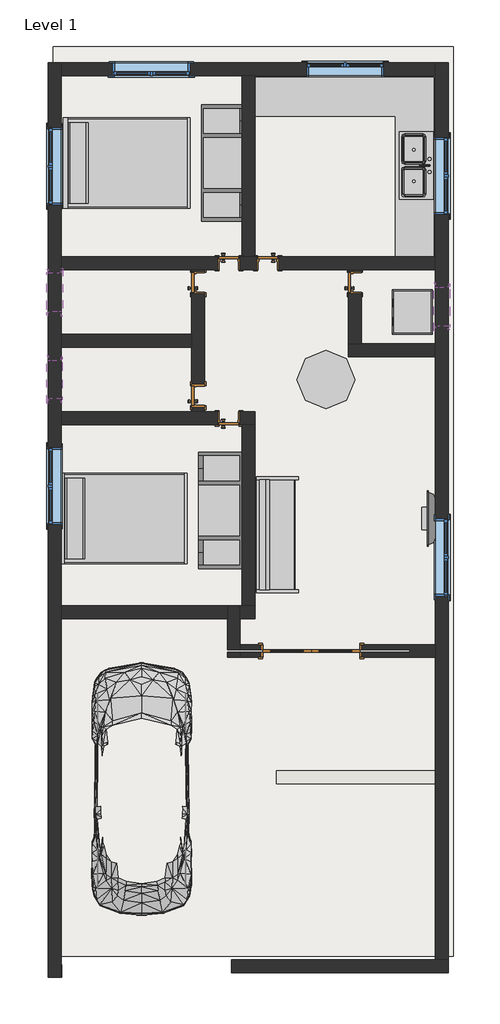
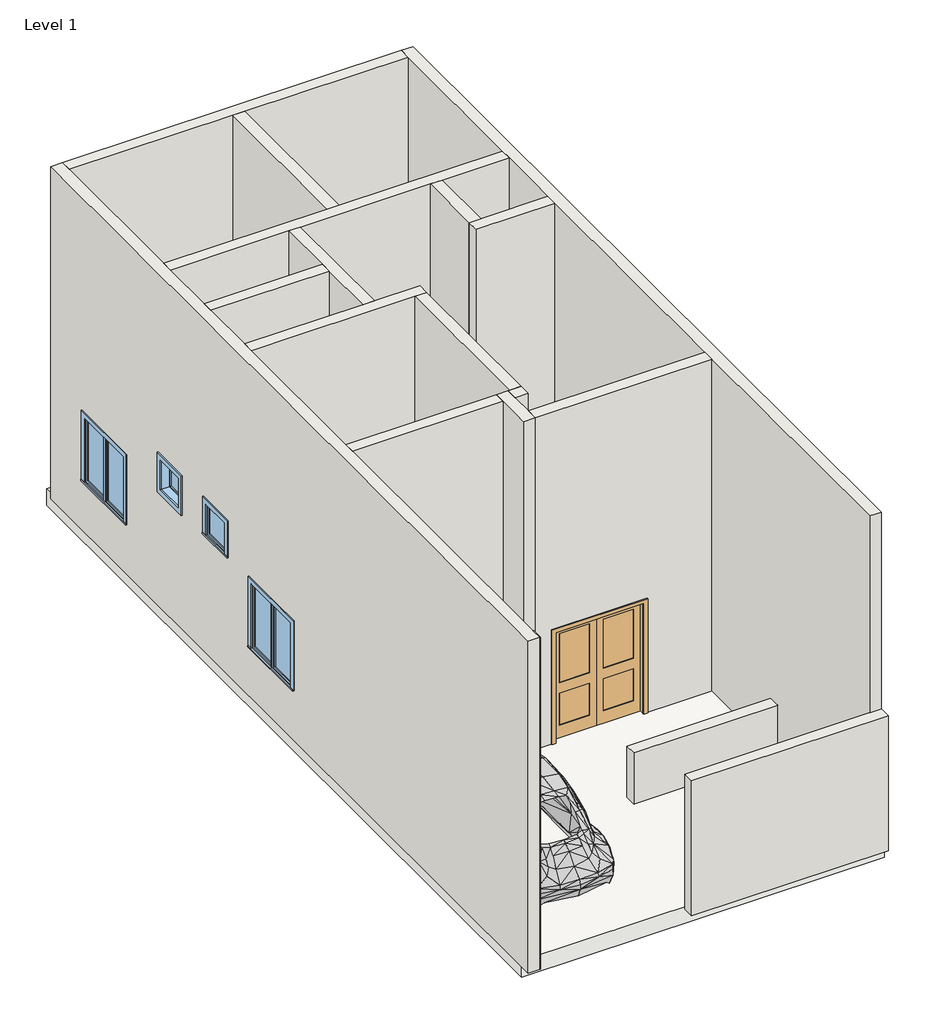
# One storey, incomplete: 17 walls, 9 windows, 8 furniture elements, 7 doors, 2 proxies, 1 flow terminal, 1 slab.
"""IFC4 building model written with IfcOpenShell, lengths in millimetres."""

from ifc_helpers import new_model, si_unit, frame, origin, origin_with_axes, place, context, project, spatial, polyline, outline, extrude, faceted_brep, transform, mapped, element, save
from components import rpc_beetle_rpc_beetle_3ce7ba48, recycle_bin_square_recycle_bin_square_c944da42, door_4110a08e, door_6ef897ee, door_5a382651, door_b2d2822a, flow_terminal_a53be723, furniture_096e7f55, furniture_8bbd1b1f, furniture_cf0b6580, furniture_a4ffab56, furniture_56245f3a, furniture_905aceb5, window_0862ab64, window_e41d21a6

model = new_model("IFC4")

# Units and contexts
model_context = context("Model", 3, world=origin())
ifc_project = project(units=[si_unit("LENGTHUNIT", "METRE", prefix="MILLI")], contexts=[model_context])

# Site, building, storey
site = spatial("IfcSite", under=ifc_project)
building = spatial("IfcBuilding", under=site)
storey = spatial("IfcBuildingStorey", under=building, Name="Level 1", Elevation=0.0)

# Proxies
placement = place(None, origin())
rpc_beetle_rpc_beetle_shape = rpc_beetle_rpc_beetle_3ce7ba48(model_context)
element("IfcBuildingElementProxy", 1, Name="RPC Beetle : RPC Beetle", ObjectType="RPC Beetle : RPC Beetle", at=placement, inside=storey, context=model_context, shape_type="MappedRepresentation", body=[
    mapped(rpc_beetle_rpc_beetle_shape, transform((-7788.5254898, -14063.9920418, 0.0), x_axis=(1.0000000000000009, 0.0, 0.0), y_axis=(0.0, 1.0000000000000009, 0.0), z_axis=(0.0, 0.0, 1.0))),
])
recycle_bin_square_recycle_bin_square_shape = recycle_bin_square_recycle_bin_square_c944da42(model_context)
element("IfcBuildingElementProxy", 2, Name="Recycle Bin-Square : Recycle Bin-Square", ObjectType="Recycle Bin-Square : Recycle Bin-Square", at=placement, inside=storey, context=model_context, shape_type="MappedRepresentation", body=[
    mapped(recycle_bin_square_recycle_bin_square_shape, transform((-3537.3649135, -5332.7420418, 0.0), x_axis=(0.0, -1.0000000000000004, 0.0), y_axis=(1.0000000000000004, 0.0, 0.0), z_axis=(0.0, 0.0, 1.0))),
])

# Doors
door_shape = door_4110a08e(model_context)
element("IfcDoor", 3, ObjectType="Door-Interior-Double-Pocket-2_Panel-Wood : 60\" x 80\"", at=placement, inside=storey, context=model_context, shape_type="MappedRepresentation", body=[
    mapped(door_shape, transform((-5121.5254898, -10660.3920418, 0.0), x_axis=(1.0, 0.0, 0.0), y_axis=(0.0, 1.0, 0.0), z_axis=(0.0, 0.0, 1.0))),
])
door_2_shape = door_6ef897ee(model_context)
element("IfcDoor", 4, ObjectType="Door-Interior-Single-5_Panel_Vert-Wood : 12\" x 80\"", at=placement, inside=storey, context=model_context, shape_type="MappedRepresentation", body=[
    mapped(door_2_shape, transform((-6416.9254898, -7005.9670418, 0.0), x_axis=(1.0, 0.0, 0.0), y_axis=(0.0, 1.0, 0.0), z_axis=(0.0, 0.0, 1.0))),
])
element("IfcDoor", 5, ObjectType="Door-Interior-Single-5_Panel_Vert-Wood : 12\" x 80\"", at=placement, inside=storey, context=model_context, shape_type="MappedRepresentation", body=[
    mapped(door_2_shape, transform((-5807.3254898, -4561.2170418, 0.0), x_axis=(-1.0, 0.0, 0.0), y_axis=(0.0, -1.0, 0.0), z_axis=(0.0, 0.0, 1.0))),
])
door_3_shape = door_5a382651(model_context)
element("IfcDoor", 6, ObjectType="Door-Interior-Single-5_Panel_Vert-Wood : 12\" x 80\"", at=placement, inside=storey, context=model_context, shape_type="MappedRepresentation", body=[
    mapped(door_3_shape, transform((-6416.9254898, -4561.2170418, 0.0), x_axis=(1.0, 0.0, 0.0), y_axis=(0.0, 1.0, 0.0), z_axis=(0.0, 0.0, 1.0))),
])
door_4_shape = door_b2d2822a(model_context)
element("IfcDoor", 7, ObjectType="Door-Interior-Single-Flush_Panel-Wood : 12\" x 80\"", at=placement, inside=storey, context=model_context, shape_type="MappedRepresentation", body=[
    mapped(door_4_shape, transform((-6902.7004898, -6647.1920418, 0.0), x_axis=(0.0, 1.0, 0.0), y_axis=(-1.0, 0.0, 0.0), z_axis=(0.0, 0.0, 1.0))),
])
element("IfcDoor", 8, ObjectType="Door-Interior-Single-Flush_Panel-Wood : 12\" x 80\"", at=placement, inside=storey, context=model_context, shape_type="MappedRepresentation", body=[
    mapped(door_4_shape, transform((-6902.7004898, -4869.1920418, 0.0), x_axis=(0.0, 1.0, 0.0), y_axis=(-1.0, 0.0, 0.0), z_axis=(0.0, 0.0, 1.0))),
])
element("IfcDoor", 9, ObjectType="Door-Interior-Single-Flush_Panel-Wood : 12\" x 80\"", at=placement, inside=storey, context=model_context, shape_type="MappedRepresentation", body=[
    mapped(door_4_shape, transform((-4438.9004898, -4869.1920418, 0.0), x_axis=(0.0, 1.0, 0.0), y_axis=(-1.0, 0.0, 0.0), z_axis=(0.0, 0.0, 1.0))),
])

# Flow terminal
flow_terminal_shape = flow_terminal_a53be723(model_context)
element("IfcFlowTerminal", 10, ObjectType="Sink Kitchen-Double : 42\" x 21\"", at=placement, inside=storey, context=model_context, shape_type="MappedRepresentation", body=[
    mapped(flow_terminal_shape, transform((-3472.8708909, -3012.0028012, 0.0), x_axis=(0.0, -1.0000000000000002, 0.0), y_axis=(1.0000000000000002, 0.0, 0.0), z_axis=(0.0, 0.0, 1.0))),
])

# Furniture
furniture_shape = furniture_096e7f55(model_context)
element("IfcFurniture", 11, ObjectType="Bed-Shaker : Double 56\" x 78\"", at=placement, inside=storey, context=model_context, shape_type="MappedRepresentation", body=[
    mapped(furniture_shape, transform((-9007.7254898, -2970.5420418, 0.0), x_axis=(0.0, 1.000000000000001, 0.0), y_axis=(-1.000000000000001, 0.0, 0.0), z_axis=(0.0, 0.0, 1.0))),
])
element("IfcFurniture", 12, ObjectType="Bed-Shaker : Double 56\" x 78\"", at=placement, inside=storey, context=model_context, shape_type="MappedRepresentation", body=[
    mapped(furniture_shape, transform((-9058.5254898, -8558.5420418, 0.0), x_axis=(0.0, 1.0, 0.0), y_axis=(-1.0, 0.0, 0.0), z_axis=(0.0, 0.0, 1.0))),
])
furniture_2_shape = furniture_8bbd1b1f(model_context)
element("IfcFurniture", 13, ObjectType="Counter Top-L Shaped w Sink : 24\" Depth", at=placement, inside=storey, context=model_context, shape_type="MappedRepresentation", body=[
    mapped(furniture_2_shape, transform((-3165.7254898, -2818.4543369, 0.0), x_axis=(0.0, -1.0000000000000002, 0.0), y_axis=(1.0000000000000002, 0.0, 0.0), z_axis=(0.0, 0.0, 1.0))),
])
furniture_3_shape = furniture_cf0b6580(model_context)
element("IfcFurniture", 14, ObjectType="Entertainment Center : 72\" x 72\" x 24\"", at=placement, inside=storey, context=model_context, shape_type="MappedRepresentation", body=[
    mapped(furniture_3_shape, transform((-6112.1254898, -8450.5920418, 0.0), x_axis=(0.0, -1.0000000000000004, 0.0), y_axis=(1.0000000000000004, 0.0, 0.0), z_axis=(0.0, 0.0, 1.0))),
])
element("IfcFurniture", 15, ObjectType="Entertainment Center : 72\" x 72\" x 24\"", at=placement, inside=storey, context=model_context, shape_type="MappedRepresentation", body=[
    mapped(furniture_3_shape, transform((-6950.3254898, -2989.5920418, 0.0), x_axis=(0.0, 1.0000000000000009, 0.0), y_axis=(-1.0000000000000009, 0.0, 0.0), z_axis=(0.0, 0.0, 1.0))),
])
furniture_4_shape = furniture_a4ffab56(model_context)
element("IfcFurniture", 16, ObjectType="Sofa : 72\"", at=placement, inside=storey, context=model_context, shape_type="MappedRepresentation", body=[
    mapped(furniture_4_shape, transform((-5508.7713914, -8901.9625336, 0.0), x_axis=(0.0, 1.0, 0.0), y_axis=(-1.0, 0.0, 0.0), z_axis=(0.0, 0.0, 1.0))),
])
furniture_5_shape = furniture_56245f3a(model_context)
element("IfcFurniture", 17, ObjectType="TV - Flat Screen : 32\"", at=placement, inside=storey, context=model_context, shape_type="MappedRepresentation", body=[
    mapped(furniture_5_shape, transform((-3227.7818717, -8581.5365559, 914.4), x_axis=(0.0, -1.0000000000000024, 0.0), y_axis=(1.0000000000000024, 0.0, 0.0), z_axis=(0.0, 0.0, 1.0))),
])
furniture_6_shape = furniture_905aceb5(model_context)
element("IfcFurniture", 18, ObjectType="Table-Dining Round w Chairs : 36\" Diameter", at=placement, inside=storey, context=model_context, shape_type="MappedRepresentation", body=[
    mapped(furniture_6_shape, transform((-4996.607457, -6208.3133533, 0.0), x_axis=(1.0, 0.0, 0.0), y_axis=(0.0, 1.0, 0.0), z_axis=(0.0, 0.0, 1.0))),
])

# Slab
element("IfcSlab", 19, ObjectType="Generic - 12\"", at=placement, inside=storey, context=model_context, shape_type="SweptSolid", body=[
    extrude(outline(polyline([(-9183.9488115, -15458.8908403), (-9183.9488115, -1158.6908403), (-2884.7488115, -1158.6908403), (-2884.7488115, -15458.8908403), (-9183.9488115, -15458.8908403)])), frame((0.0, 0.0, -304.8), z_axis=(0.0, 0.0, 1.0), x_axis=(1.0, 0.0, 0.0)), (0.0, 0.0, 1.0), 304.8),
])

# Walls
element("IfcWall", 20, ObjectType="Generic - 8\"", at=placement, inside=storey, context=model_context, shape_type="Brep", body=[
    faceted_brep([(-9058.5254898, -15791.1920418, 0.0), (-9058.5254898, -15587.9920418, 0.0), (-9058.5254898, -10152.3920418, 0.0), (-9058.5254898, -9949.1920418, 0.0), (-9058.5254898, -7104.3920418, 0.0), (-9058.5254898, -6901.1920418, 0.0), (-9058.5254898, -5885.1920418, 0.0), (-9058.5254898, -5681.9920418, 0.0), (-9058.5254898, -4665.9920418, 0.0), (-9058.5254898, -4462.7920418, 0.0), (-9058.5254898, -1617.9920418, 0.0), (-9058.5254898, -1414.7920418, 0.0), (-9058.5254898, -1414.7920418, 6096.0), (-9058.5254898, -1617.9920418, 6096.0), (-9058.5254898, -4462.7920418, 6096.0), (-9058.5254898, -4665.9920418, 6096.0), (-9058.5254898, -5681.9920418, 6096.0), (-9058.5254898, -5885.1920418, 6096.0), (-9058.5254898, -6901.1920418, 6096.0), (-9058.5254898, -7104.3920418, 6096.0), (-9058.5254898, -9949.1920418, 6096.0), (-9058.5254898, -10152.3920418, 6096.0), (-9058.5254898, -15587.9920418, 6096.0), (-9058.5254898, -15791.1920418, 6096.0), (-9058.5254898, -7459.9920418, 2133.6), (-9058.5254898, -7459.9920418, 914.4), (-9058.5254898, -8679.1920418, 914.4), (-9058.5254898, -8679.1920418, 2133.6), (-9058.5254898, -2430.7920418, 2133.6), (-9058.5254898, -2430.7920418, 914.4), (-9058.5254898, -3649.9920418, 914.4), (-9058.5254898, -3649.9920418, 2133.6), (-9058.5254898, -6088.3920418, 2768.6), (-9058.5254898, -6088.3920418, 2159.0), (-9058.5254898, -6697.9920418, 2159.0), (-9058.5254898, -6697.9920418, 2768.6), (-9058.5254898, -5326.3920418, 2768.6), (-9058.5254898, -4716.7920418, 2768.6), (-9058.5254898, -4716.7920418, 2159.0), (-9058.5254898, -5326.3920418, 2159.0), (-9261.7254898, -15791.1920418, 0.0), (-9261.7254898, -15791.1920418, 6096.0), (-9261.7254898, -1414.7920418, 6096.0), (-9261.7254898, -1414.7920418, 0.0), (-9261.7254898, -7459.9920418, 2133.6), (-9261.7254898, -8679.1920418, 2133.6), (-9261.7254898, -8679.1920418, 914.4), (-9261.7254898, -7459.9920418, 914.4), (-9261.7254898, -2430.7920418, 2133.6), (-9261.7254898, -3649.9920418, 2133.6), (-9261.7254898, -3649.9920418, 914.4), (-9261.7254898, -2430.7920418, 914.4), (-9261.7254898, -6088.3920418, 2768.6), (-9261.7254898, -6697.9920418, 2768.6), (-9261.7254898, -6697.9920418, 2159.0), (-9261.7254898, -6088.3920418, 2159.0), (-9261.7254898, -5326.3920418, 2768.6), (-9261.7254898, -5326.3920418, 2159.0), (-9261.7254898, -4716.7920418, 2159.0), (-9261.7254898, -4716.7920418, 2768.6)], [[[0, 1, 2, 3, 4, 5, 6, 7, 8, 9, 10, 11, 12, 13, 14, 15, 16, 17, 18, 19, 20, 21, 22, 23], [24, 25, 26, 27], [28, 29, 30, 31], [32, 33, 34, 35], [36, 37, 38, 39]], [[40, 41, 42, 43], [44, 45, 46, 47], [48, 49, 50, 51], [52, 53, 54, 55], [56, 57, 58, 59]], [[11, 10, 9, 8, 7, 6, 5, 4, 3, 2, 1, 0, 40, 43]], [[23, 22, 21, 20, 19, 18, 17, 16, 15, 14, 13, 12, 42, 41]], [[12, 11, 43, 42]], [[0, 23, 41, 40]], [[25, 24, 44, 47]], [[26, 25, 47, 46]], [[27, 26, 46, 45]], [[24, 27, 45, 44]], [[29, 28, 48, 51]], [[30, 29, 51, 50]], [[31, 30, 50, 49]], [[28, 31, 49, 48]], [[33, 32, 52, 55]], [[34, 33, 55, 54]], [[35, 34, 54, 53]], [[32, 35, 53, 52]], [[57, 56, 36, 39]], [[58, 57, 39, 38]], [[59, 58, 38, 37]], [[56, 59, 37, 36]]]),
])
element("IfcWall", 21, ObjectType="Generic - 8\"", at=placement, inside=storey, context=model_context, shape_type="Brep", body=[
    faceted_brep([(-9058.5254898, -1617.9920418, 0.0), (-6213.7254898, -1617.9920418, 0.0), (-6010.5254898, -1617.9920418, 0.0), (-3165.7254898, -1617.9920418, 0.0), (-3165.7254898, -1617.9920418, 6096.0), (-6010.5254898, -1617.9920418, 6096.0), (-6213.7254898, -1617.9920418, 6096.0), (-9058.5254898, -1617.9920418, 6096.0), (-8245.7254898, -1617.9920418, 2133.6), (-7026.5254898, -1617.9920418, 2133.6), (-7026.5254898, -1617.9920418, 914.4), (-8245.7254898, -1617.9920418, 914.4), (-3978.5254898, -1617.9920418, 2133.6), (-3978.5254898, -1617.9920418, 914.4), (-5197.7254898, -1617.9920418, 914.4), (-5197.7254898, -1617.9920418, 2133.6), (-9058.5254898, -1414.7920418, 0.0), (-9058.5254898, -1414.7920418, 6096.0), (-3165.7254898, -1414.7920418, 6096.0), (-3165.7254898, -1414.7920418, 0.0), (-8245.7254898, -1414.7920418, 2133.6), (-8245.7254898, -1414.7920418, 914.4), (-7026.5254898, -1414.7920418, 914.4), (-7026.5254898, -1414.7920418, 2133.6), (-3978.5254898, -1414.7920418, 2133.6), (-5197.7254898, -1414.7920418, 2133.6), (-5197.7254898, -1414.7920418, 914.4), (-3978.5254898, -1414.7920418, 914.4)], [[[0, 1, 2, 3, 4, 5, 6, 7], [8, 9, 10, 11], [12, 13, 14, 15]], [[16, 17, 18, 19], [20, 21, 22, 23], [24, 25, 26, 27]], [[3, 2, 1, 0, 16, 19]], [[7, 6, 5, 4, 18, 17]], [[0, 7, 17, 16]], [[4, 3, 19, 18]], [[21, 20, 8, 11]], [[22, 21, 11, 10]], [[23, 22, 10, 9]], [[20, 23, 9, 8]], [[13, 12, 24, 27]], [[14, 13, 27, 26]], [[15, 14, 26, 25]], [[12, 15, 25, 24]]]),
])
element("IfcWall", 22, ObjectType="Generic - 8\"", at=placement, inside=storey, context=model_context, shape_type="Brep", body=[
    faceted_brep([(-3165.7254898, -1414.7920418, 0.0), (-3165.7254898, -1617.9920418, 0.0), (-3165.7254898, -4462.7920418, 0.0), (-3165.7254898, -4665.9920418, 0.0), (-3165.7254898, -5834.3920418, 0.0), (-3165.7254898, -6037.5920418, 0.0), (-3165.7254898, -10558.7920418, 0.0), (-3165.7254898, -10761.9920418, 0.0), (-3165.7254898, -15511.7920418, 0.0), (-3165.7254898, -15511.7920418, 6096.0), (-3165.7254898, -10761.9920418, 6096.0), (-3165.7254898, -10558.7920418, 6096.0), (-3165.7254898, -6037.5920418, 6096.0), (-3165.7254898, -5834.3920418, 6096.0), (-3165.7254898, -4665.9920418, 6096.0), (-3165.7254898, -4462.7920418, 6096.0), (-3165.7254898, -1617.9920418, 6096.0), (-3165.7254898, -1414.7920418, 6096.0), (-3165.7254898, -9796.7920418, 2133.6), (-3165.7254898, -9796.7920418, 914.4), (-3165.7254898, -8577.5920418, 914.4), (-3165.7254898, -8577.5920418, 2133.6), (-3165.7254898, -3802.3920418, 2133.6), (-3165.7254898, -3802.3920418, 914.4), (-3165.7254898, -2583.1920418, 914.4), (-3165.7254898, -2583.1920418, 2133.6), (-3165.7254898, -4945.3920418, 2768.6), (-3165.7254898, -5554.9920418, 2768.6), (-3165.7254898, -5554.9920418, 2159.0), (-3165.7254898, -4945.3920418, 2159.0), (-2962.5254898, -1414.7920418, 0.0), (-2962.5254898, -1414.7920418, 6096.0), (-2962.5254898, -15511.7920418, 6096.0), (-2962.5254898, -15511.7920418, 2479.6226957), (-2962.5254898, -15511.7920418, 0.0), (-2962.5254898, -9796.7920418, 2133.6), (-2962.5254898, -8577.5920418, 2133.6), (-2962.5254898, -8577.5920418, 914.4), (-2962.5254898, -9796.7920418, 914.4), (-2962.5254898, -3802.3920418, 2133.6), (-2962.5254898, -2583.1920418, 2133.6), (-2962.5254898, -2583.1920418, 914.4), (-2962.5254898, -3802.3920418, 914.4), (-2962.5254898, -4945.3920418, 2768.6), (-2962.5254898, -4945.3920418, 2159.0), (-2962.5254898, -5554.9920418, 2159.0), (-2962.5254898, -5554.9920418, 2768.6)], [[[0, 1, 2, 3, 4, 5, 6, 7, 8, 9, 10, 11, 12, 13, 14, 15, 16, 17], [18, 19, 20, 21], [22, 23, 24, 25], [26, 27, 28, 29]], [[30, 31, 32, 33, 34], [35, 36, 37, 38], [39, 40, 41, 42], [43, 44, 45, 46]], [[8, 7, 6, 5, 4, 3, 2, 1, 0, 30, 34]], [[17, 16, 15, 14, 13, 12, 11, 10, 9, 32, 31]], [[0, 17, 31, 30]], [[9, 8, 34, 33, 32]], [[19, 18, 35, 38]], [[20, 19, 38, 37]], [[21, 20, 37, 36]], [[18, 21, 36, 35]], [[23, 22, 39, 42]], [[24, 23, 42, 41]], [[25, 24, 41, 40]], [[22, 25, 40, 39]], [[44, 43, 26, 29]], [[45, 44, 29, 28]], [[46, 45, 28, 27]], [[43, 46, 27, 26]]]),
])
element("IfcWall", 23, ObjectType="Generic - 8\"", at=placement, inside=storey, context=model_context, shape_type="Brep", body=[
    faceted_brep([(-2962.5254898, -15511.7920418, 0.0), (-3165.7254898, -15511.7920418, 0.0), (-6378.8254898, -15511.7920418, 0.0), (-6378.8254898, -15511.7920418, 2479.6226957), (-2962.5254898, -15511.7920418, 2479.6226957), (-2962.5254898, -15714.9920418, 0.0), (-2962.5254898, -15714.9920418, 2479.6226957), (-6378.8254898, -15714.9920418, 2479.6226957), (-6378.8254898, -15714.9920418, 0.0)], [[[0, 1, 2, 3, 4]], [[5, 6, 7, 8]], [[2, 1, 0, 5, 8]], [[3, 2, 8, 7]], [[4, 3, 7, 6]], [[0, 4, 6, 5]]]),
])
element("IfcWall", 24, ObjectType="Generic - 8\"", at=placement, inside=storey, context=model_context, shape_type="Brep", body=[
    faceted_brep([(-3165.7254898, -4665.9920418, 6096.0), (-4334.1254898, -4665.9920418, 6096.0), (-4537.3254898, -4665.9920418, 6096.0), (-6797.9254898, -4665.9920418, 6096.0), (-7001.1254898, -4665.9920418, 6096.0), (-9058.5254898, -4665.9920418, 6096.0), (-9058.5254898, -4665.9920418, 0.0), (-7001.1254898, -4665.9920418, 0.0), (-6797.9254898, -4665.9920418, 0.0), (-6594.7254898, -4665.9920418, 0.0), (-6594.7254898, -4665.9920418, 2057.4), (-6239.1254898, -4665.9920418, 2057.4), (-6239.1254898, -4665.9920418, 0.0), (-5985.1254898, -4665.9920418, 0.0), (-5985.1254898, -4665.9920418, 2057.4), (-5629.5254898, -4665.9920418, 2057.4), (-5629.5254898, -4665.9920418, 0.0), (-4537.3254898, -4665.9920418, 0.0), (-4334.1254898, -4665.9920418, 0.0), (-3165.7254898, -4665.9920418, 0.0), (-9058.5254898, -4462.7920418, 6096.0), (-6213.7254898, -4462.7920418, 6096.0), (-6010.5254898, -4462.7920418, 6096.0), (-3165.7254898, -4462.7920418, 6096.0), (-3165.7254898, -4462.7920418, 0.0), (-5629.5254898, -4462.7920418, 0.0), (-5629.5254898, -4462.7920418, 2057.4), (-5985.1254898, -4462.7920418, 2057.4), (-5985.1254898, -4462.7920418, 0.0), (-6010.5254898, -4462.7920418, 0.0), (-6213.7254898, -4462.7920418, 0.0), (-6239.1254898, -4462.7920418, 0.0), (-6239.1254898, -4462.7920418, 2057.4), (-6594.7254898, -4462.7920418, 2057.4), (-6594.7254898, -4462.7920418, 0.0), (-9058.5254898, -4462.7920418, 0.0)], [[[0, 1, 2, 3, 4, 5, 6, 7, 8, 9, 10, 11, 12, 13, 14, 15, 16, 17, 18, 19]], [[20, 21, 22, 23, 24, 25, 26, 27, 28, 29, 30, 31, 32, 33, 34, 35]], [[6, 35, 34, 9, 8, 7]], [[24, 19, 18, 17, 16, 25]], [[12, 31, 30, 29, 28, 13]], [[5, 4, 3, 2, 1, 0, 23, 22, 21, 20]], [[6, 5, 20, 35]], [[0, 19, 24, 23]], [[11, 32, 31, 12]], [[32, 11, 10, 33]], [[33, 10, 9, 34]], [[27, 14, 13, 28]], [[14, 27, 26, 15]], [[15, 26, 25, 16]]]),
])
element("IfcWall", 25, ObjectType="Generic - 8\"", at=placement, inside=storey, context=model_context, shape_type="SweptSolid", body=[
    extrude(outline(polyline([(-6010.5254898, -1617.9920418), (-6010.5254898, -4462.7920418), (-6213.7254898, -4462.7920418), (-6213.7254898, -1617.9920418), (-6010.5254898, -1617.9920418)])), origin_with_axes(), (0.0, 0.0, 1.0), 6096.0),
])
element("IfcWall", 26, ObjectType="Generic - 8\"", at=placement, inside=storey, context=model_context, shape_type="SweptSolid", body=[
    extrude(outline(polyline([(-7001.1254898, -5885.1920418), (-9058.5254898, -5885.1920418), (-9058.5254898, -5681.9920418), (-7001.1254898, -5681.9920418), (-7001.1254898, -5885.1920418)])), origin_with_axes(), (0.0, 0.0, 1.0), 6096.0),
])
element("IfcWall", 27, ObjectType="Generic - 8\"", at=placement, inside=storey, context=model_context, shape_type="Brep", body=[
    faceted_brep([(-6010.5254898, -7104.3920418, 6096.0), (-6213.7254898, -7104.3920418, 6096.0), (-9058.5254898, -7104.3920418, 6096.0), (-9058.5254898, -7104.3920418, 0.0), (-6594.7254898, -7104.3920418, 0.0), (-6594.7254898, -7104.3920418, 2057.4), (-6239.1254898, -7104.3920418, 2057.4), (-6239.1254898, -7104.3920418, 0.0), (-6213.7254898, -7104.3920418, 0.0), (-6010.5254898, -7104.3920418, 0.0), (-9058.5254898, -6901.1920418, 6096.0), (-7001.1254898, -6901.1920418, 6096.0), (-6797.9254898, -6901.1920418, 6096.0), (-6010.5254898, -6901.1920418, 6096.0), (-6010.5254898, -6901.1920418, 0.0), (-6239.1254898, -6901.1920418, 0.0), (-6239.1254898, -6901.1920418, 2057.4), (-6594.7254898, -6901.1920418, 2057.4), (-6594.7254898, -6901.1920418, 0.0), (-6797.9254898, -6901.1920418, 0.0), (-7001.1254898, -6901.1920418, 0.0), (-9058.5254898, -6901.1920418, 0.0)], [[[0, 1, 2, 3, 4, 5, 6, 7, 8, 9]], [[10, 11, 12, 13, 14, 15, 16, 17, 18, 19, 20, 21]], [[3, 21, 20, 19, 18, 4]], [[14, 9, 8, 7, 15]], [[2, 1, 0, 13, 12, 11, 10]], [[3, 2, 10, 21]], [[0, 9, 14, 13]], [[6, 16, 15, 7]], [[16, 6, 5, 17]], [[17, 5, 4, 18]]]),
])
element("IfcWall", 28, ObjectType="Generic - 8\"", at=placement, inside=storey, context=model_context, shape_type="Brep", body=[
    faceted_brep([(-9058.5254898, -10152.3920418, 6096.0), (-9058.5254898, -10152.3920418, 0.0), (-6442.3254898, -10152.3920418, 0.0), (-6442.3254898, -10152.3920418, 6096.0), (-9058.5254898, -9949.1920418, 0.0), (-9058.5254898, -9949.1920418, 6096.0), (-6442.3254898, -9949.1920418, 6096.0), (-6442.3254898, -9949.1920418, 0.0)], [[[0, 1, 2, 3]], [[4, 5, 6, 7]], [[1, 4, 7, 2]], [[5, 0, 3, 6]], [[1, 0, 5, 4]], [[3, 2, 7, 6]]]),
    faceted_brep([(-6010.5254898, -10152.3920418, 0.0), (-6010.5254898, -10152.3920418, 6096.0), (-6239.1254898, -10152.3920418, 6096.0), (-6239.1254898, -10152.3920418, 0.0), (-6010.5254898, -9949.1920418, 6096.0), (-6010.5254898, -9949.1920418, 0.0), (-6213.7254898, -9949.1920418, 0.0), (-6239.1254898, -9949.1920418, 0.0), (-6239.1254898, -9949.1920418, 6096.0), (-6213.7254898, -9949.1920418, 6096.0)], [[[0, 1, 2, 3]], [[4, 5, 6, 7, 8, 9]], [[5, 0, 3, 7, 6]], [[1, 4, 9, 8, 2]], [[1, 0, 5, 4]], [[3, 2, 8, 7]]]),
])
element("IfcWall", 29, ObjectType="Generic - 8\"", at=placement, inside=storey, context=model_context, shape_type="SweptSolid", body=[
    extrude(outline(polyline([(-5667.6254898, -12539.9920418), (-3165.7254898, -12539.9920418), (-3165.7254898, -12743.1920418), (-5667.6254898, -12743.1920418), (-5667.6254898, -12539.9920418)])), frame((0.0, 0.0, -120.3257282), z_axis=(0.0, 0.0, 1.0), x_axis=(1.0, 0.0, 0.0)), (0.0, 0.0, 1.0), 1063.7134836),
])
element("IfcWall", 30, ObjectType="Generic - 8\"", at=placement, inside=storey, context=model_context, shape_type="Brep", body=[
    faceted_brep([(-6239.1254898, -10558.7920418, 6096.0), (-3165.7254898, -10558.7920418, 6096.0), (-3165.7254898, -10558.7920418, 0.0), (-4334.1254898, -10558.7920418, 0.0), (-4334.1254898, -10558.7920418, 2057.4), (-5908.9254898, -10558.7920418, 2057.4), (-5908.9254898, -10558.7920418, 0.0), (-6239.1254898, -10558.7920418, 0.0), (-3165.7254898, -10761.9920418, 6096.0), (-6239.1254898, -10761.9920418, 6096.0), (-6239.1254898, -10761.9920418, 0.0), (-5908.9254898, -10761.9920418, 0.0), (-5908.9254898, -10761.9920418, 2057.4), (-4334.1254898, -10761.9920418, 2057.4), (-4334.1254898, -10761.9920418, 0.0), (-3165.7254898, -10761.9920418, 0.0), (-4334.1254898, -10681.0295418, 0.0), (-3572.1254898, -10681.0295418, 0.0), (-3572.1254898, -10639.7545418, 0.0), (-4334.1254898, -10639.7545418, 0.0), (-5908.9254898, -10639.7545418, 0.0), (-6239.1254898, -10639.7545418, 0.0), (-6239.1254898, -10681.0295418, 0.0), (-5908.9254898, -10681.0295418, 0.0), (-6239.1254898, -10639.7545418, 2057.4), (-6239.1254898, -10681.0295418, 2057.4), (-3572.1254898, -10639.7545418, 2057.4), (-3572.1254898, -10681.0295418, 2057.4), (-4334.1254898, -10681.0295418, 2057.4), (-5908.9254898, -10681.0295418, 2057.4), (-5908.9254898, -10639.7545418, 2057.4), (-4334.1254898, -10639.7545418, 2057.4)], [[[0, 1, 2, 3, 4, 5, 6, 7]], [[8, 9, 10, 11, 12, 13, 14, 15]], [[2, 15, 14, 16, 17, 18, 19, 3]], [[7, 6, 20, 21]], [[11, 10, 22, 23]], [[1, 0, 9, 8]], [[2, 1, 8, 15]], [[0, 7, 21, 24, 25, 22, 10, 9]], [[26, 27, 28, 13, 12, 29, 25, 24, 30, 5, 4, 31]], [[26, 31, 19, 18]], [[31, 4, 3, 19]], [[5, 30, 20, 6]], [[20, 30, 24, 21]], [[29, 23, 22, 25]], [[29, 12, 11, 23]], [[13, 28, 16, 14]], [[28, 27, 17, 16]], [[27, 26, 18, 17]]]),
])
element("IfcWall", 31, ObjectType="Generic - 8\"", at=placement, inside=storey, context=model_context, shape_type="Brep", body=[
    faceted_brep([(-4537.3254898, -6037.5920418, 0.0), (-3165.7254898, -6037.5920418, 0.0), (-3165.7254898, -6037.5920418, 6096.0), (-4537.3254898, -6037.5920418, 6096.0), (-4537.3254898, -5834.3920418, 0.0), (-4537.3254898, -5834.3920418, 6096.0), (-4334.1254898, -5834.3920418, 6096.0), (-3165.7254898, -5834.3920418, 6096.0), (-3165.7254898, -5834.3920418, 0.0), (-4334.1254898, -5834.3920418, 0.0)], [[[0, 1, 2, 3]], [[4, 5, 6, 7, 8, 9]], [[1, 0, 4, 9, 8]], [[3, 2, 7, 6, 5]], [[2, 1, 8, 7]], [[0, 3, 5, 4]]]),
])
element("IfcWall", 32, ObjectType="Generic - 8\"", at=placement, inside=storey, context=model_context, shape_type="SweptSolid", body=[
    extrude(outline(polyline([(-5834.3920418, 6096.0), (-4665.9920418, 6096.0), (-4665.9920418, 0.0), (-4691.3920418, 0.0), (-4691.3920418, 2057.4), (-5046.9920418, 2057.4), (-5046.9920418, 0.0), (-5834.3920418, 0.0), (-5834.3920418, 6096.0)])), frame((-4537.3254898, 0.0, 0.0), z_axis=(1.0, 0.0, 0.0), x_axis=(0.0, 1.0, 0.0)), (0.0, 0.0, 1.0), 203.2),
])
element("IfcWall", 33, ObjectType="Generic - 8\"", at=placement, inside=storey, context=model_context, shape_type="SweptSolid", body=[
    extrude(outline(polyline([(-6010.5254898, -7104.3920418), (-6010.5254898, -9949.1920418), (-6213.7254898, -9949.1920418), (-6213.7254898, -7104.3920418), (-6010.5254898, -7104.3920418)])), origin_with_axes(), (0.0, 0.0, 1.0), 6096.0),
])
element("IfcWall", 34, ObjectType="Generic - 8\"", at=placement, inside=storey, context=model_context, shape_type="Brep", body=[
    faceted_brep([(-6797.9254898, -4665.9920418, 0.0), (-6797.9254898, -4665.9920418, 6096.0), (-6797.9254898, -6901.1920418, 6096.0), (-6797.9254898, -6901.1920418, 0.0), (-6797.9254898, -6824.9920418, 0.0), (-6797.9254898, -6824.9920418, 2057.4), (-6797.9254898, -6469.3920418, 2057.4), (-6797.9254898, -6469.3920418, 0.0), (-6797.9254898, -5046.9920418, 0.0), (-6797.9254898, -5046.9920418, 2057.4), (-6797.9254898, -4691.3920418, 2057.4), (-6797.9254898, -4691.3920418, 0.0), (-7001.1254898, -4665.9920418, 6096.0), (-7001.1254898, -4665.9920418, 0.0), (-7001.1254898, -4691.3920418, 0.0), (-7001.1254898, -4691.3920418, 2057.4), (-7001.1254898, -5046.9920418, 2057.4), (-7001.1254898, -5046.9920418, 0.0), (-7001.1254898, -5681.9920418, 0.0), (-7001.1254898, -5885.1920418, 0.0), (-7001.1254898, -6469.3920418, 0.0), (-7001.1254898, -6469.3920418, 2057.4), (-7001.1254898, -6824.9920418, 2057.4), (-7001.1254898, -6824.9920418, 0.0), (-7001.1254898, -6901.1920418, 0.0), (-7001.1254898, -6901.1920418, 6096.0), (-7001.1254898, -5885.1920418, 6096.0), (-7001.1254898, -5681.9920418, 6096.0)], [[[0, 1, 2, 3, 4, 5, 6, 7, 8, 9, 10, 11]], [[12, 13, 14, 15, 16, 17, 18, 19, 20, 21, 22, 23, 24, 25, 26, 27]], [[13, 0, 11, 14]], [[7, 20, 19, 18, 17, 8]], [[23, 4, 3, 24]], [[1, 12, 27, 26, 25, 2]], [[1, 0, 13, 12]], [[3, 2, 25, 24]], [[6, 21, 20, 7]], [[21, 6, 5, 22]], [[22, 5, 4, 23]], [[10, 15, 14, 11]], [[15, 10, 9, 16]], [[16, 9, 8, 17]]]),
])
element("IfcWall", 35, ObjectType="Generic - 8\"", at=placement, inside=storey, context=model_context, shape_type="Brep", body=[
    faceted_brep([(-6239.1254898, -9949.1920418, 0.0), (-6239.1254898, -9949.1920418, 6096.0), (-6239.1254898, -10152.3920418, 6096.0), (-6239.1254898, -10558.7920418, 6096.0), (-6239.1254898, -10761.9920418, 6096.0), (-6239.1254898, -10761.9920418, 0.0), (-6239.1254898, -10681.0295418, 0.0), (-6239.1254898, -10681.0295418, 2057.4), (-6239.1254898, -10639.7545418, 2057.4), (-6239.1254898, -10639.7545418, 0.0), (-6239.1254898, -10558.7920418, 0.0), (-6239.1254898, -10152.3920418, 0.0), (-6442.3254898, -9949.1920418, 6096.0), (-6442.3254898, -9949.1920418, 0.0), (-6442.3254898, -10152.3920418, 0.0), (-6442.3254898, -10639.7545418, 0.0), (-6442.3254898, -10639.7545418, 2057.4), (-6442.3254898, -10681.0295418, 2057.4), (-6442.3254898, -10681.0295418, 0.0), (-6442.3254898, -10761.9920418, 0.0), (-6442.3254898, -10761.9920418, 6096.0), (-6442.3254898, -10152.3920418, 6096.0)], [[[0, 1, 2, 3, 4, 5, 6, 7, 8, 9, 10, 11]], [[12, 13, 14, 15, 16, 17, 18, 19, 20, 21]], [[13, 0, 11, 10, 9, 15, 14]], [[5, 19, 18, 6]], [[1, 0, 13, 12]], [[4, 3, 2, 1, 12, 21, 20]], [[5, 4, 20, 19]], [[7, 17, 16, 8]], [[8, 16, 15, 9]], [[17, 7, 6, 18]]]),
])
element("IfcWall", 36, ObjectType="Generic - 8\"", at=placement, inside=storey, context=model_context, shape_type="SweptSolid", body=[
    extrude(outline(polyline([(-9058.5254898, -15587.9920418), (-9045.8254898, -15587.9920418), (-9045.8254898, -15791.1920418), (-9058.5254898, -15791.1920418), (-9058.5254898, -15587.9920418)])), origin_with_axes(), (0.0, 0.0, 1.0), 6096.0),
])

# Windows
window_shape = window_0862ab64(model_context)
element("IfcWindow", 37, ObjectType="Casement Dbl with Trim : 48\" x 48\"", at=placement, inside=storey, context=model_context, shape_type="MappedRepresentation", body=[
    mapped(window_shape, transform((-3083.1754898, -9187.1920418, 0.0), x_axis=(0.0, -1.0, 0.0), y_axis=(1.0, 0.0, 0.0), z_axis=(0.0, 0.0, 1.0))),
])
element("IfcWindow", 38, ObjectType="Casement Dbl with Trim : 48\" x 48\"", at=placement, inside=storey, context=model_context, shape_type="MappedRepresentation", body=[
    mapped(window_shape, transform((-3083.1754898, -3192.7920418, 0.0), x_axis=(0.0, -1.0, 0.0), y_axis=(1.0, 0.0, 0.0), z_axis=(0.0, 0.0, 1.0))),
])
element("IfcWindow", 39, ObjectType="Casement Dbl with Trim : 48\" x 48\"", at=placement, inside=storey, context=model_context, shape_type="MappedRepresentation", body=[
    mapped(window_shape, transform((-9141.0754898, -8069.5920418, 0.0), x_axis=(0.0, 1.0, 0.0), y_axis=(-1.0, 0.0, 0.0), z_axis=(0.0, 0.0, 1.0))),
])
element("IfcWindow", 40, ObjectType="Casement Dbl with Trim : 48\" x 48\"", at=placement, inside=storey, context=model_context, shape_type="MappedRepresentation", body=[
    mapped(window_shape, transform((-9141.0754898, -3040.3920418, 0.0), x_axis=(0.0, 1.0, 0.0), y_axis=(-1.0, 0.0, 0.0), z_axis=(0.0, 0.0, 1.0))),
])
element("IfcWindow", 41, ObjectType="Casement Dbl with Trim : 48\" x 48\"", at=placement, inside=storey, context=model_context, shape_type="MappedRepresentation", body=[
    mapped(window_shape, transform((-7636.1254898, -1497.3420418, 0.0), x_axis=(-1.0, 0.0, 0.0), y_axis=(0.0, -1.0, 0.0), z_axis=(0.0, 0.0, 1.0))),
])
element("IfcWindow", 42, ObjectType="Casement Dbl with Trim : 48\" x 48\"", at=placement, inside=storey, context=model_context, shape_type="MappedRepresentation", body=[
    mapped(window_shape, transform((-4588.1254898, -1535.4420418, 0.0), x_axis=(1.0, 0.0, 0.0), y_axis=(0.0, 1.0, 0.0), z_axis=(0.0, 0.0, 1.0))),
])
window_2_shape = window_e41d21a6(model_context)
element("IfcWindow", 43, ObjectType="Transom with Trim : 24\" x 24\"", at=placement, inside=storey, context=model_context, shape_type="MappedRepresentation", body=[
    mapped(window_2_shape, transform((-9160.1254898, -6355.0920418, 0.0), x_axis=(0.0, 1.0, 0.0), y_axis=(-1.0, 0.0, 0.0), z_axis=(0.0, 0.0, 1.0))),
])
element("IfcWindow", 44, ObjectType="Transom with Trim : 24\" x 24\"", at=placement, inside=storey, context=model_context, shape_type="MappedRepresentation", body=[
    mapped(window_2_shape, transform((-9160.1254898, -5059.6920418, 0.0), x_axis=(0.0, -1.0, 0.0), y_axis=(1.0, 0.0, 0.0), z_axis=(0.0, 0.0, 1.0))),
])
element("IfcWindow", 45, ObjectType="Transom with Trim : 24\" x 24\"", at=placement, inside=storey, context=model_context, shape_type="MappedRepresentation", body=[
    mapped(window_2_shape, transform((-3064.1254898, -5212.0920418, 0.0), x_axis=(0.0, 1.0, 0.0), y_axis=(-1.0, 0.0, 0.0), z_axis=(0.0, 0.0, 1.0))),
])

save(model, "model.ifc")

# Revit data of these elements
# Type "RPC Beetle : RPC Beetle"
#   built-in parameter 1005195 = "RPC-16-0U6E-L4EG-ENH1-J3KF-SVEL-0TX4-C0"
#   Height = 0
# Type "Recycle Bin-Square : Recycle Bin-Square"
#   Default Elevation = 0
# Type "Door-Interior-Double-Pocket-2_Panel-Wood : 60\" x 80\""
#   Type Mark = "11"
#   Assembly Code = "C1020300"
#   Analytic Construction = "Wooden"
#   Top Rail = 0' - 4 11/16"
#   Thickness = 0' - 1 3/8"
#   Thermal Resistance (R) = 2.5876 (h·ft²·°F)/BTU
#   Stiles = 0' - 4 3/4"
#   Rough Width = 10' - 2"
#   Rough Height = 7' - 0 1/2"
#   Panel Width = 2' - 6"
#   Lock Rail = 0' - 7 1/2"
#   Location [instance default] = 2' - 7"
#   Height = 6' - 8"
#   Width = 5' - 0"
#   Heat Transfer Coefficient (U) = 0.3865 BTU/(h·ft²·°F)
#   Bottom Rail = 0' - 9 1/8"
#   Panel Open [instance default] = no
#   Trim Material = Cherry
#   Panel Material = Cherry
#   Frame Material = Cherry
#   Visual Light Transmittance = 0
#   Solar Heat Gain Coefficient = 0
#   Wall Closure = (empty or 0)
#   Function = (empty or 0)
# Type "Door-Interior-Single-5_Panel_Vert-Wood : 12\" x 80\""
#   Type Mark = "8"
#   Assembly Code = "C1020300"
#   Analytic Construction = "Wooden"
#   Top Rail = 0' - 4 11/16"
#   Thickness = 0' - 1 3/8"
#   Thermal Resistance (R) = 2.5876 (h·ft²·°F)/BTU
#   Swing Angle [instance default] = 90.00°
#   Stiles = 0' - 2 3/8"
#   Rough Width = 1' - 2"
#   Rough Height = 6' - 9"
#   Intermediate Rail = 0' - 4 1/2"
#   Height = 6' - 8"
#   Width = 1' - 0"
#   Heat Transfer Coefficient (U) = 0.3865 BTU/(h·ft²·°F)
#   Bottom Rail = 0' - 9 1/8"
#   Trim Material = Cherry
#   Panel Material = Cherry
#   Frame Material = Cherry
#   Door Handle Material = Aluminum
#   Visual Light Transmittance = 0
#   Solar Heat Gain Coefficient = 0
#   Wall Closure = (empty or 0)
#   Function = (empty or 0)
# Type "Door-Interior-Single-Flush_Panel-Wood : 12\" x 80\""
#   Type Mark = "10"
#   Assembly Code = "C1020300"
#   Analytic Construction = "Wooden"
#   Thickness = 0' - 1 3/8"
#   Thermal Resistance (R) = 2.5876 (h·ft²·°F)/BTU
#   Swing Angle [instance default] = 90.00°
#   Rough Width = 1' - 2"
#   Rough Height = 6' - 9"
#   Height = 6' - 8"
#   Width = 1' - 0"
#   Heat Transfer Coefficient (U) = 0.3865 BTU/(h·ft²·°F)
#   Trim Material = Cherry
#   Panel Material = Cherry
#   Frame Material = Cherry
#   Door Handle Material = Aluminum
#   Visual Light Transmittance = 0
#   Solar Heat Gain Coefficient = 0
#   Wall Closure = (empty or 0)
#   Function = (empty or 0)
# Type "Sink Kitchen-Double : 42\" x 21\""
#   Assembly Code = "D2010410"
#   Counter Height = 3' - 0"
#   Depth = 1' - 9"
#   Width = 3' - 6"
#   Faucet Material = Steel, Polished
#   Sink Material = Steel, Polished
#   Default Elevation = 0
# Type "Bed-Shaker : Double 56\" x 78\""
#   Assembly Code = "E2020200"
#   Length = 6' - 6"
#   Width = 4' - 8"
#   Frame Material = Birch
#   Mattress Material = Linen, White
#   Default Elevation = 0
# Type "Counter Top-L Shaped w Sink : 24\" Depth"
#   Assembly Code = "C1030400"
#   Counter Thickness = 0' - 1 1/2"
#   Depth = 2' - 1"
#   Height = 3' - 0"
#   Length - Leg 1 [instance default] = 8' - 0"
#   Length - Leg 2 [instance default] = 6' - 0"
#   Sink Location [instance default] = 3' - 0"
#   Sink Location To Wall [instance default] = 0' - 6"
#   Sink Opening Depth [instance default] = 1' - 3"
#   Sink Opening Width [instance default] = 3' - 3"
#   Counter Top Material = none
#   Default Elevation = 0
# Type "Entertainment Center : 72\" x 72\" x 24\""
#   Assembly Code = "E2020200"
#   Center Width = 2' - 8"
#   Depth = 2' - 0"
#   Height = 6' - 0"
#   Width = 6' - 0"
#   Material = none
#   Default Elevation = 0
# Type "Sofa : 72\""
#   Assembly Code = "E2020200"
#   Width = 6' - 0"
#   Seat Material = Linen, Beige
#   Frame Material = Cherry
#   Default Elevation = 0
# Type "TV - Flat Screen : 32\""
#   SinAng = 0' - 0.0193"
#   L = 2' - 3.79372"
#   H = 1' - 3.6354"
#   Thickness = 0' - 4.33071"
#   Diagonal = 2' - 7.88976"
#   CosAng = 0' - 0.03431"
#   Stand [instance default] = yes
#   Default Elevation = 0
# Type "Table-Dining Round w Chairs : 36\" Diameter"
#   Assembly Code = "E2020200"
#   Radius = 1' - 6"
#   Diameter = 3' - 0"
#   Height = 2' - 6"
#   Chairs = 4
#   Base Material = Pine
#   Top Material = Laminate, Linen, Matte
#   Default Elevation = 0
# Type "Generic - 12\""
#   Assembly Code = "B1010"
#   Function = 0
#   Layers, outside or top first: 1' - 0" no material (function 1)
# Type "Generic - 8\""
#   Assembly Code = "B2010"
#   Layers, outside or top first: 0' - 8" "Default Mass Interior Wall" (function 1)
# Type "Casement Dbl with Trim : 48\" x 48\""
#   Type Mark = "10"
#   Construction Type Id = "GSP4R"
#   Assembly Code = "B2020100"
#   Analytic Construction = "1/8 in Pilkington single glazing"
#   Visual Light Transmittance = 0.9
#   Solar Heat Gain Coefficient = 0.78
#   Heat Transfer Coefficient (U) = 0.6496 BTU/(h·ft²·°F)
#   Height = 4' - 0"
#   Default Sill Height = 3' - 0"
#   Trim Projection - Ext. = 0' - 0 1/2"
#   Trim Projection - Int. = 0' - 0 3/4"
#   Trim Width - Exterior = 0' - 3 1/2"
#   Trim Width - Interior = 0' - 3 1/2"
#   Width = 4' - 0"
#   Window Inset = 0' - 0 3/4"
#   Define Thermal Properties by = 1
#   Glass Pane Material = Glass
#   Sash Material = Sash
#   Trim Exterior Material = Trim
#   Trim Interior Material = Trim
#   Wall Closure = (empty or 0)
# Type "Transom with Trim : 24\" x 24\""
#   Type Mark = "13"
#   Construction Type Id = "GSP4R"
#   Assembly Code = "B2020100"
#   Analytic Construction = "1/8 in Pilkington single glazing"
#   Visual Light Transmittance = 0.9
#   Solar Heat Gain Coefficient = 0.78
#   Heat Transfer Coefficient (U) = 0.6496 BTU/(h·ft²·°F)
#   Height = 2' - 0"
#   Default Sill Height = 7' - 1"
#   Trim Projection - Ext. = 0' - 0 1/2"
#   Trim Projection - Int. = 0' - 0 3/4"
#   Trim Width - Exterior = 0' - 3 1/2"
#   Trim Width - Interior = 0' - 3 1/2"
#   Width = 2' - 0"
#   Window Inset = 0' - 0 3/4"
#   Define Thermal Properties by = 1
#   Glass Pane Material = Glass
#   Sash Material = Sash
#   Trim Exterior Material = Trim
#   Trim Interior Material = Trim
#   Wall Closure = (empty or 0)
# Element 1 (IfcBuildingElementProxy, "RPC Beetle : RPC Beetle")
#   Phase Created = New Construction
# Element 2 (IfcBuildingElementProxy, "Recycle Bin-Square : Recycle Bin-Square")
#   Phase Created = New Construction
#   Materials on its faces: "Plastic - Blue", "Default - Black"
# Element 3 (IfcDoor, "Door-Interior-Double-Pocket-2_Panel-Wood : 60\" x 80\"")
#   Location = 2' - 7"
#   Panel Open = no
#   Phase Created = New Construction
#   Materials on its faces: "Cherry"
# Elements 4, 5, 6 (IfcDoor, "Door-Interior-Single-5_Panel_Vert-Wood : 12\" x 80\"")
#   Swing Angle = 90.00°
#   Phase Created = New Construction
#   Materials on its faces: "Cherry", "Aluminum"
# Elements 7, 8, 9 (IfcDoor, "Door-Interior-Single-Flush_Panel-Wood : 12\" x 80\"")
#   Swing Angle = 90.00°
#   Phase Created = New Construction
#   Materials on its faces: "Cherry", "Aluminum"
# Element 10 (IfcFlowTerminal, "Sink Kitchen-Double : 42\" x 21\"")
#   Mark = "4"
#   Phase Created = New Construction
#   Materials on its faces: "Steel, Polished"
# Elements 11, 12 (IfcFurniture, "Bed-Shaker : Double 56\" x 78\"")
#   Phase Created = New Construction
#   Materials on its faces: "Birch", "Linen, White"
# Element 13 (IfcFurniture, "Counter Top-L Shaped w Sink : 24\" Depth")
#   Sink Opening Width = 3' - 3"
#   Sink Opening Depth = 1' - 3"
#   Sink Location To Wall = 0' - 6"
#   Sink Location = 3' - 0"
#   Length - Leg 2 = 9' - 4"
#   Length - Leg 1 = 9' - 4"
#   Phase Created = New Construction
#   Materials on its faces: "Counter Top"
# Elements 14, 15 (IfcFurniture, "Entertainment Center : 72\" x 72\" x 24\"")
#   Phase Created = New Construction
#   Materials on its faces: "Steel, Chrome Plated", "Glass - Clear, Grey"
# Element 16 (IfcFurniture, "Sofa : 72\"")
#   Phase Created = New Construction
#   Materials on its faces: "Cherry", "Linen, Beige"
# Element 17 (IfcFurniture, "TV - Flat Screen : 32\"")
#   Stand = yes
#   Phase Created = New Construction
#   Materials on its faces: "TV - Black", "TV - Glass", "TV - Screen"
# Element 18 (IfcFurniture, "Table-Dining Round w Chairs : 36\" Diameter")
#   Phase Created = New Construction
#   Materials on its faces: "Pine", "Laminate, Linen, Matte"
# Element 19 (IfcSlab, "Generic - 12\"")
#   built-in parameter 1001955 = -1.5708 (stored number, unit not read)
#   Height Offset From Level = 0' - 0"
#   Phase Created = New Construction
#   Materials on its faces: "Default Floor"
# Elements 20, 21, 22, 24, 25, 26, 27, 28, 30, 31, 32, 33, 34, 35, 36 (IfcWall, "Generic - 8\"")
#   Top Offset = 0' - 0"
#   Base Offset = 0' - 0"
#   Unconnected Height = 20' - 0"
#   wall height = 20' - 0"
#   Phase Created = New Construction
#   Base Constraint = Level 1
#   Materials on its faces: "Default Mass Interior Wall"
# Element 23 (IfcWall, "Generic - 8\"")
#   Top Offset = 0' - 0"
#   Base Offset = 0' - 0"
#   Unconnected Height = 8' - 1.62294"
#   wall height = 8' - 1.62294"
#   Phase Created = New Construction
#   Base Constraint = Level 1
#   Materials on its faces: "Default Mass Interior Wall"
# Element 29 (IfcWall, "Generic - 8\"")
#   built-in parameter 1001111 = -0' - 4.73723"
#   Top Offset = 0' - 0"
#   Base Offset = -0' - 4.73723"
#   Unconnected Height = 3' - 5.87848"
#   wall height = 3' - 5.87848"
#   Phase Created = New Construction
#   Base Constraint = Level 1
#   Materials on its faces: "Default Mass Interior Wall"
# Element 37 (IfcWindow, "Casement Dbl with Trim : 48\" x 48\"")
#   Mark = "1"
#   Phase Created = New Construction
#   Materials on its faces: "Sash", "Trim", "Glass"
# Element 38 (IfcWindow, "Casement Dbl with Trim : 48\" x 48\"")
#   Mark = "2"
#   Phase Created = New Construction
#   Materials on its faces: "Sash", "Trim", "Glass"
# Element 39 (IfcWindow, "Casement Dbl with Trim : 48\" x 48\"")
#   Mark = "3"
#   Phase Created = New Construction
#   Materials on its faces: "Sash", "Trim", "Glass"
# Element 40 (IfcWindow, "Casement Dbl with Trim : 48\" x 48\"")
#   Mark = "4"
#   Phase Created = New Construction
#   Materials on its faces: "Sash", "Trim", "Glass"
# Element 41 (IfcWindow, "Casement Dbl with Trim : 48\" x 48\"")
#   Mark = "5"
#   Phase Created = New Construction
#   Materials on its faces: "Sash", "Trim", "Glass"
# Element 42 (IfcWindow, "Casement Dbl with Trim : 48\" x 48\"")
#   Mark = "6"
#   Phase Created = New Construction
#   Materials on its faces: "Sash", "Trim", "Glass"
# Element 43 (IfcWindow, "Transom with Trim : 24\" x 24\"")
#   Mark = "7"
#   Phase Created = New Construction
#   Materials on its faces: "Sash", "Trim", "Glass"
# Element 44 (IfcWindow, "Transom with Trim : 24\" x 24\"")
#   Mark = "8"
#   Phase Created = New Construction
#   Materials on its faces: "Sash", "Trim", "Glass"
# Element 45 (IfcWindow, "Transom with Trim : 24\" x 24\"")
#   Mark = "9"
#   Phase Created = New Construction
#   Materials on its faces: "Sash", "Trim", "Glass"
# Materials
#   "Cherry": class "Wood", colour RGB 226 177 128, transparency 0, Description = "Prunus Serotina", Cost = 0
#   "Aluminum": class "Metal", colour RGB 247 247 247, transparency 0, Description = "Aluminum 6061", Cost = 0
#   "Steel, Polished": class "Metal", colour RGB 57 57 57, transparency 0, Description = "Polished steel", Cost = 0
#   "Birch": class "Wood", colour RGB 224 178 126, transparency 0, Description = "Betula Alleghaniensis", Cost = 0
#   "Linen, White": class "Textile", colour RGB 247 247 239, transparency 0, Description = "Linen, white", Cost = 0
#   "Linen, Beige": class "Textile", colour RGB 249 239 230, transparency 0, Description = "Linen, beige", Cost = 0
#   "Pine": class "Wood", colour RGB 223 192 134, transparency 0, Description = "Pinus Echinata", Cost = 0
#   "Laminate, Linen, Matte": class "Plastic", colour RGB 249 239 230, transparency 0, Description = "Plastic Laminate - Linen, Matte", Cost = 0
#   "Default Mass Interior Wall": class "Generic", colour RGB 195 229 126, transparency 0, Cost = 0
#   "Glass": class "Glass", colour RGB 0 128 192, transparency 0.75, Description = "Soda Lime Glass", Cost = 0
#   "Sash": class "Wood", colour RGB 224 178 126, transparency 0
#   "Trim": class "Wood", colour RGB 224 178 126, transparency 0
#   "Plastic - Blue": class "Plastic", colour RGB 0 0 212, transparency 0
#   "Default - Black": colour RGB 0 0 0, transparency 0
#   "Counter Top": class "Wood", colour RGB 226 177 128, transparency 0
#   "Steel, Chrome Plated": class "Metal", colour RGB 17 17 17, transparency 0, Description = "Chromiuim plated steel", Cost = 0
#   "Glass - Clear, Grey": class "Glass", colour RGB 252 255 255, transparency 0.64
#   "TV - Black": colour RGB 49 49 49, transparency 0
#   "TV - Glass": colour RGB 157 157 157, transparency 0.9
#   "TV - Screen": colour RGB 0 0 0, transparency 0
#   "Default Floor": colour RGB 128 128 128, transparency 0
